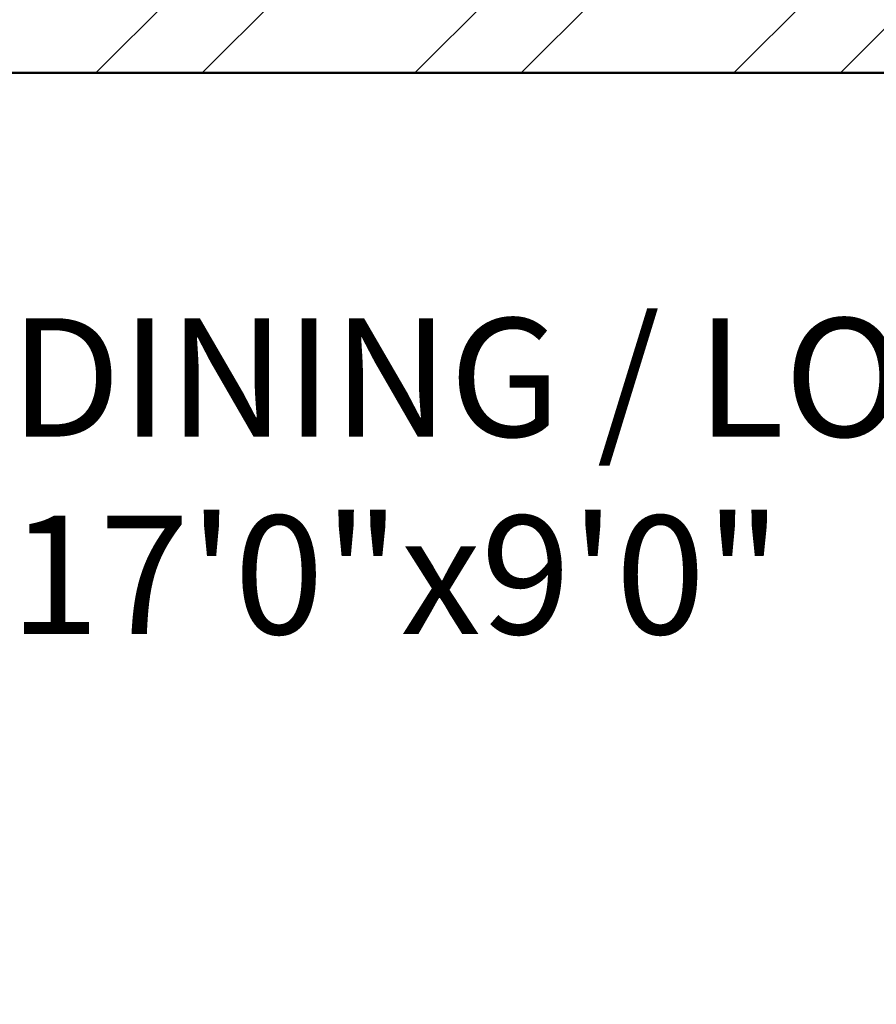
# Model space of a CAD drawing. Units: inches. Extents: x 963 to 2075, y 289 to 2657.
# Tile 63 of 98: x 1188 to 1224, y 2284 to 2325. Entities that reach past the tile are written whole.
import ezdxf

# ---------------------------------------------------------------- set-up
doc = ezdxf.new("R2010")
doc.units = ezdxf.units.IN
for name, color, linetype, lineweight in [('A-AREA-IDEN', 7, 'Continuous', 18), ('A-WALL', 7, 'Continuous', 50), ('A-WALL-PATT', 8, 'Continuous', 13)]:
    doc.layers.add(name, color=color, linetype=linetype, lineweight=lineweight)
doc.styles.get("Standard").update_dxf_attribs({"font": 'arial.ttf'})

msp = doc.modelspace()

# ---------------------------------------------------------------- hatches: boundary and pattern name
at = {"layer": 'A-WALL-PATT'}
h = msp.add_hatch(dxfattribs=at)
h.set_pattern_fill('ANSI32', color=256)
h.paths.add_polyline_path([(1296.922, 2558.318), (1203.922, 2558.318), (1203.922, 2493.818), (1191.533, 2493.818), (1191.533, 2489.318), (1211.063, 2489.318), (1211.063, 2492.02), (1211.063, 2493.818), (1208.422, 2493.818), (1208.422, 2553.818), (1292.422, 2553.818), (1292.422, 2538.863), (1296.922, 2538.863)])
h.paths.add_polyline_path([(1442.422, 2558.318), (1349.422, 2558.318), (1349.422, 2538.943), (1353.922, 2538.943), (1353.922, 2553.818), (1437.922, 2553.818), (1437.922, 2493.818), (1434.542, 2493.818), (1434.542, 2489.318), (1448.311, 2489.318), (1448.311, 2491.568), (1448.311, 2493.818), (1442.422, 2493.818)])
h.paths.add_polyline_path([(1415.554, 2491.568), (1415.554, 2493.818), (1340.941, 2493.818), (1340.941, 2489.318), (1371.922, 2489.318), (1371.922, 2378.318), (1367.596, 2378.318), (1367.596, 2373.818), (1371.922, 2373.818), (1371.922, 2355.185), (1376.422, 2355.185), (1376.422, 2489.318), (1415.554, 2489.318)])
h.paths.add_polyline_path([(1304.941, 2491.568), (1304.941, 2493.818), (1296.922, 2493.818), (1296.922, 2514.863), (1292.422, 2514.863), (1292.422, 2493.818), (1232.808, 2493.818), (1232.808, 2489.318), (1256.422, 2489.318), (1256.422, 2327.318), (1253.714, 2327.318), (1253.714, 2322.818), (1328.422, 2322.818), (1328.422, 2331.147), (1323.922, 2331.147), (1323.922, 2327.318), (1260.922, 2327.318), (1260.922, 2373.818), (1323.922, 2373.818), (1323.922, 2357.812), (1328.422, 2357.812), (1328.422, 2373.818), (1346.007, 2373.818), (1346.007, 2376.068), (1346.007, 2378.318), (1260.922, 2378.318), (1260.922, 2489.318), (1304.941, 2489.318)])
h.paths.add_polyline_path([(1226.654, 2327.318), (1124.422, 2327.318), (1124.422, 2347.447), (1119.922, 2347.447), (1119.922, 2322.818), (1163.422, 2322.818), (1163.422, 2305.435), (1165.672, 2305.435), (1167.922, 2305.435), (1167.922, 2322.818), (1226.654, 2322.818), (1226.654, 2325.068)])
h.paths.add_polyline_path([(1095.922, 2489.318), (1124.422, 2489.318), (1131.533, 2489.318), (1131.533, 2491.568), (1131.533, 2493.818), (1119.922, 2493.818), (1091.422, 2493.818), (1091.422, 2417.318), (1095.922, 2417.318), (1119.922, 2417.318), (1119.922, 2407.447), (1124.422, 2407.447), (1124.422, 2421.818), (1095.922, 2421.818)])
h.paths.add_polyline_path([(1512.922, 2558.318), (1508.422, 2558.318), (1508.422, 2493.818), (1503.401, 2493.818), (1503.401, 2489.318), (1508.422, 2489.318), (1508.422, 2327.318), (1376.422, 2327.318), (1376.422, 2330.273), (1371.922, 2330.273), (1371.922, 2298.744), (1376.422, 2298.744), (1376.422, 2322.818), (1508.422, 2322.818), (1508.422, 2165.318), (1504.255, 2165.318), (1504.255, 2160.818), (1508.422, 2160.818), (1508.422, 2108.318), (1512.922, 2108.318), (1512.922, 2160.818), (1516.182, 2160.818), (1516.182, 2163.068), (1516.182, 2165.318), (1512.922, 2165.318), (1512.922, 2322.818), (1644.922, 2322.818), (1644.922, 2298.744), (1649.422, 2298.744), (1649.422, 2322.818), (1649.422, 2330.944), (1647.172, 2330.944), (1644.922, 2330.944), (1644.922, 2327.318), (1512.922, 2327.318), (1512.922, 2489.318), (1516.759, 2489.318), (1516.759, 2491.568), (1516.759, 2493.818), (1512.922, 2493.818)])
h.paths.add_polyline_path([(1671.922, 2558.318), (1578.922, 2558.318), (1578.922, 2493.818), (1573.526, 2493.818), (1573.526, 2489.318), (1586.537, 2489.318), (1586.537, 2491.568), (1586.537, 2493.818), (1583.422, 2493.818), (1583.422, 2553.818), (1667.422, 2553.818), (1667.422, 2541.109), (1671.922, 2541.109)])
h.paths.add_polyline_path([(1681.257, 2493.818), (1671.922, 2493.818), (1671.922, 2517.109), (1667.422, 2517.109), (1667.422, 2493.818), (1610.218, 2493.818), (1610.218, 2489.318), (1644.922, 2489.318), (1644.922, 2357.865), (1649.422, 2357.865), (1649.422, 2373.818), (1652.203, 2373.818), (1652.203, 2375.827), (1652.203, 2378.318), (1649.422, 2378.318), (1649.422, 2489.318), (1681.257, 2489.318), (1681.257, 2491.568)])
h.paths.add_polyline_path([(1821.922, 2558.318), (1728.922, 2558.318), (1728.922, 2541), (1733.422, 2541), (1733.422, 2553.818), (1817.422, 2553.818), (1817.422, 2493.818), (1813.507, 2493.818), (1813.507, 2489.318), (1830.078, 2489.318), (1830.078, 2491.568), (1830.078, 2493.818), (1821.922, 2493.818)])
h.paths.add_polyline_path([(1794.244, 2493.818), (1717.257, 2493.818), (1717.257, 2489.318), (1760.422, 2489.318), (1760.422, 2378.318), (1674.401, 2378.318), (1674.401, 2373.818), (1692.922, 2373.818), (1692.922, 2356.954), (1697.422, 2356.954), (1697.422, 2373.818), (1760.422, 2373.818), (1760.422, 2327.318), (1697.422, 2327.318), (1697.422, 2333.341), (1692.922, 2333.341), (1692.922, 2322.818), (1768.037, 2322.818), (1768.037, 2325.068), (1768.037, 2327.318), (1764.922, 2327.318), (1764.922, 2489.318), (1794.244, 2489.318)])
h.paths.add_polyline_path([(1733.422, 2517), (1728.922, 2517), (1728.922, 2493.818), (1733.422, 2493.818)], flags=17)
h.paths.add_polyline_path([(1929.922, 2493.818), (1890.078, 2493.818), (1890.078, 2489.318), (1896.922, 2489.318), (1925.422, 2489.318), (1925.422, 2421.818), (1896.922, 2421.818), (1896.922, 2408.318), (1901.422, 2408.318), (1901.422, 2417.318), (1925.422, 2417.318), (1929.922, 2417.318)])
h.paths.add_polyline_path([(1901.422, 2348.318), (1896.922, 2348.318), (1896.922, 2327.318), (1800.423, 2327.318), (1800.423, 2322.818), (1853.422, 2322.818), (1853.422, 2309.453), (1857.922, 2309.453), (1857.922, 2322.818), (1901.422, 2322.818)])
h.paths.add_polyline_path([(1857.922, 2249.453), (1853.422, 2249.453), (1853.422, 2214.818), (1686.309, 2214.818), (1686.309, 2210.318), (1853.422, 2210.318), (1853.422, 2202.134), (1857.922, 2202.134), (1857.922, 2210.318)])
h.paths.add_polyline_path([(1857.922, 2142.134), (1853.422, 2142.134), (1853.422, 2115.422), (1841.422, 2115.422), (1841.422, 2088.531), (1841.422, 2046.949), (1845.922, 2046.949), (1845.922, 2110.922), (1905.922, 2110.922), (1905.922, 2092.517), (1910.422, 2092.517), (1910.422, 2115.422), (1857.922, 2115.422)])
h.paths.add_polyline_path([(1532.436, 1482.342), (1573.456, 1482.342), (1573.456, 1501), (1532.436, 1501)], flags=9)
h.paths.add_polyline_path([(1438.658, 1486.302), (1479.678, 1486.302), (1479.678, 1504.96), (1438.658, 1504.96)], flags=9)
h.paths.add_polyline_path([(1411.215, 1365.308), (1659.139, 1365.308), (1659.139, 1402.401), (1411.215, 1402.401)], flags=9)
h.paths.add_polyline_path([(1185.671, 2296.298), (1248.16, 2296.298), (1248.16, 2314.955), (1185.671, 2314.955)], flags=9)
h.paths.add_polyline_path([(1177.31, 2187.35), (1216.15, 2187.35), (1216.15, 2206.007), (1177.31, 2206.007)], flags=9)
h.paths.add_polyline_path([(1295.101, 1602.083), (1328.26, 1602.083), (1328.26, 1620.741), (1295.101, 1620.741)], flags=9)
h.paths.add_polyline_path([(1525.126, 2005.99), (1558.39, 2005.99), (1558.39, 2024.648), (1525.126, 2024.648)], flags=9)
h.paths.add_polyline_path([(1459.606, 1977.125), (1472.195, 1977.125), (1472.195, 1987.429), (1459.606, 1987.429)], flags=9)
h.paths.add_polyline_path([(1467.815, 2053.676), (1480.018, 2053.676), (1480.018, 2063.979), (1467.815, 2063.979)], flags=9)
h.paths.add_polyline_path([(1555.184, 2119.02), (1584.563, 2119.02), (1584.563, 2137.678), (1555.184, 2137.678)], flags=25)
h.paths.add_polyline_path([(1405.389, 2115.291), (1444.478, 2115.291), (1444.478, 2133.948), (1405.389, 2133.948)], flags=25)
h.paths.add_polyline_path([(1698.482, 2004.259), (1727.695, 2004.259), (1727.695, 2022.916), (1698.482, 2022.916)], flags=9)
h.paths.add_polyline_path([(1612.158, 1972.855), (1629.016, 1972.855), (1629.016, 1983.159), (1612.158, 1983.159)], flags=9)
h.paths.add_polyline_path([(1608.289, 2060.036), (1625.147, 2060.036), (1625.147, 2070.34), (1608.289, 2070.34)], flags=9)
h.paths.add_polyline_path([(1527.954, 1684.402), (1566.795, 1684.402), (1566.795, 1703.06), (1527.954, 1703.06)], flags=9)
h.paths.add_polyline_path([(1422.792, 1683.59), (1461.633, 1683.59), (1461.633, 1702.247), (1422.792, 1702.247)], flags=9)
h.paths.add_polyline_path([(1531.262, 1732.459), (1574.015, 1732.459), (1574.015, 1751.116), (1531.262, 1751.116)], flags=9)
h.paths.add_polyline_path([(1402.872, 1732.845), (1439.799, 1732.845), (1439.799, 1751.502), (1402.872, 1751.502)], flags=9)
h.paths.add_polyline_path([(1243.122, 1923.132), (1281.962, 1923.132), (1281.962, 1941.79), (1243.122, 1941.79)], flags=9)
h.paths.add_polyline_path([(1181.752, 1792.268), (1244.241, 1792.268), (1244.241, 1810.926), (1181.752, 1810.926)], flags=9)
h.paths.add_polyline_path([(1265.822, 1670.3), (1316.071, 1670.3), (1316.071, 1688.957), (1265.822, 1688.957)], flags=9)
h.paths.add_polyline_path([(1140.263, 1676.054), (1179.104, 1676.054), (1179.104, 1694.711), (1140.263, 1694.711)], flags=9)
h.paths.add_polyline_path([(1107.49, 1490.889), (1143.374, 1490.889), (1143.374, 1509.546), (1107.49, 1509.546)], flags=9)
h.paths.add_polyline_path([(1217.584, 1483.899), (1246.741, 1483.899), (1246.741, 1502.556), (1217.584, 1502.556)], flags=9)
h.paths.add_polyline_path([(1389.21, 1486.919), (1418.367, 1486.919), (1418.367, 1505.576), (1389.21, 1505.576)], flags=9)
h.paths.add_polyline_path([(1672.208, 1602.083), (1705.366, 1602.083), (1705.366, 1620.741), (1672.208, 1620.741)], flags=9)
h.paths.add_polyline_path([(1752.082, 1522.638), (1781.24, 1522.638), (1781.24, 1541.295), (1752.082, 1541.295)], flags=9)
h.paths.add_polyline_path([(1848.275, 1491.26), (1884.158, 1491.26), (1884.158, 1509.918), (1848.275, 1509.918)], flags=9)
h.paths.add_polyline_path([(1822.47, 1685.62), (1861.31, 1685.62), (1861.31, 1704.278), (1822.47, 1704.278)], flags=9)
h.paths.add_polyline_path([(1713.195, 1672.232), (1763.444, 1672.232), (1763.444, 1690.889), (1713.195, 1690.889)], flags=9)
h.paths.add_polyline_path([(1736.619, 1790.578), (1799.109, 1790.578), (1799.109, 1809.235), (1736.619, 1809.235)], flags=9)
h.paths.add_polyline_path([(1691.491, 1916.355), (1730.332, 1916.355), (1730.332, 1935.013), (1691.491, 1935.013)], flags=9)
h.paths.add_polyline_path([(1764.872, 1973.922), (1794.306, 1973.922), (1794.306, 1992.58), (1764.872, 1992.58)], flags=9)
h.paths.add_polyline_path([(1767.854, 2034.017), (1797.288, 2034.017), (1797.288, 2052.674), (1767.854, 2052.674)], flags=9)
h.paths.add_polyline_path([(1851.593, 2060.331), (1880.751, 2060.331), (1880.751, 2078.989), (1851.593, 2078.989)], flags=25)
h.paths.add_polyline_path([(1688.491, 2086.874), (1727.332, 2086.874), (1727.332, 2105.531), (1688.491, 2105.531)], flags=9)
h.paths.add_polyline_path([(1537.743, 2293.581), (1580.495, 2293.581), (1580.495, 2312.239), (1537.743, 2312.239)], flags=25)
h.paths.add_polyline_path([(1425.587, 2296.109), (1468.34, 2296.109), (1468.34, 2314.766), (1425.587, 2314.766)], flags=25)
h.paths.add_polyline_path([(1278.518, 2004.184), (1307.72, 2004.184), (1307.72, 2022.841), (1278.518, 2022.841)], flags=9)
h.paths.add_polyline_path([(1193.282, 1973.635), (1222.715, 1973.635), (1222.715, 1992.292), (1193.282, 1992.292)], flags=9)
h.paths.add_polyline_path([(1192.411, 2040.577), (1221.845, 2040.577), (1221.845, 2059.234), (1192.411, 2059.234)], flags=9)
h.paths.add_polyline_path([(1130.603, 1951.393), (1159.76, 1951.393), (1159.76, 1970.05), (1130.603, 1970.05)], flags=9)
h.paths.add_polyline_path([(1132.827, 2052.494), (1161.984, 2052.494), (1161.984, 2071.151), (1132.827, 2071.151)], flags=9)
h.paths.add_polyline_path([(1265.128, 2334.619), (1315.377, 2334.619), (1315.377, 2353.277), (1265.128, 2353.277)], flags=25)
h.paths.add_polyline_path([(1136.741, 2330.785), (1175.582, 2330.785), (1175.582, 2349.443), (1136.741, 2349.443)], flags=9)
h.paths.add_polyline_path([(1287.422, 2417.204), (1320.58, 2417.204), (1320.58, 2435.861), (1287.422, 2435.861)], flags=25)
h.paths.add_polyline_path([(1430.988, 2329.159), (1469.828, 2329.159), (1469.828, 2347.816), (1430.988, 2347.816)], flags=25)
h.paths.add_polyline_path([(1525.424, 2329.213), (1564.264, 2329.213), (1564.264, 2347.87), (1525.424, 2347.87)], flags=25)
h.paths.add_polyline_path([(1684.525, 2382.799), (1717.683, 2382.799), (1717.683, 2401.457), (1684.525, 2401.457)], flags=25)
h.paths.add_polyline_path([(1704.805, 2340.293), (1755.054, 2340.293), (1755.054, 2358.95), (1704.805, 2358.95)], flags=25)
h.paths.add_polyline_path([(1694.113, 2287.757), (1756.602, 2287.757), (1756.602, 2306.414), (1694.113, 2306.414)], flags=9)
h.paths.add_polyline_path([(1815.778, 2329.861), (1854.618, 2329.861), (1854.618, 2348.518), (1815.778, 2348.518)], flags=9)
h.paths.add_polyline_path([(1842.873, 2514.256), (1878.756, 2514.256), (1878.756, 2532.914), (1842.873, 2532.914)], flags=9)
h.paths.add_polyline_path([(1769.513, 2531.447), (1798.671, 2531.447), (1798.671, 2550.104), (1769.513, 2550.104)], flags=25)
h.paths.add_polyline_path([(1594.772, 2518.468), (1623.93, 2518.468), (1623.93, 2537.125), (1594.772, 2537.125)], flags=25)
h.paths.add_polyline_path([(1520.723, 2516.185), (1556.606, 2516.185), (1556.606, 2534.842), (1520.723, 2534.842)], flags=25)
h.paths.add_polyline_path([(1464.456, 2516.694), (1500.34, 2516.694), (1500.34, 2535.351), (1464.456, 2535.351)], flags=25)
h.paths.add_polyline_path([(1365.696, 2528.97), (1394.854, 2528.97), (1394.854, 2547.627), (1365.696, 2547.627)], flags=25)
h.paths.add_polyline_path([(1222.838, 2516.231), (1251.995, 2516.231), (1251.995, 2534.889), (1222.838, 2534.889)], flags=25)
h.paths.add_polyline_path([(1104.545, 2509.6), (1140.429, 2509.6), (1140.429, 2528.257), (1104.545, 2528.257)], flags=9)
h = msp.add_hatch(dxfattribs=at)
h.set_pattern_fill('ANSI32', color=256)
h.paths.add_polyline_path([(1335.968, 2212.568), (1335.968, 2214.818), (1167.922, 2214.818), (1167.922, 2245.435), (1163.422, 2245.435), (1163.422, 2210.318), (1163.422, 2194.812), (1167.922, 2194.812), (1167.922, 2210.318), (1335.968, 2210.318)])
h.paths.add_polyline_path([(1532.436, 1482.342), (1573.456, 1482.342), (1573.456, 1501), (1532.436, 1501)], flags=9)
h.paths.add_polyline_path([(1438.658, 1486.302), (1479.678, 1486.302), (1479.678, 1504.96), (1438.658, 1504.96)], flags=9)
h.paths.add_polyline_path([(1411.215, 1365.308), (1659.139, 1365.308), (1659.139, 1402.401), (1411.215, 1402.401)], flags=9)
h.paths.add_polyline_path([(1185.671, 2296.298), (1248.16, 2296.298), (1248.16, 2314.955), (1185.671, 2314.955)], flags=9)
h.paths.add_polyline_path([(1177.31, 2187.35), (1216.15, 2187.35), (1216.15, 2206.007), (1177.31, 2206.007)], flags=9)
h.paths.add_polyline_path([(1295.101, 1602.083), (1328.26, 1602.083), (1328.26, 1620.741), (1295.101, 1620.741)], flags=9)
h.paths.add_polyline_path([(1525.126, 2005.99), (1558.39, 2005.99), (1558.39, 2024.648), (1525.126, 2024.648)], flags=9)
h.paths.add_polyline_path([(1459.606, 1977.125), (1472.195, 1977.125), (1472.195, 1987.429), (1459.606, 1987.429)], flags=9)
h.paths.add_polyline_path([(1467.815, 2053.676), (1480.018, 2053.676), (1480.018, 2063.979), (1467.815, 2063.979)], flags=9)
h.paths.add_polyline_path([(1555.184, 2119.02), (1584.563, 2119.02), (1584.563, 2137.678), (1555.184, 2137.678)], flags=9)
h.paths.add_polyline_path([(1405.389, 2115.291), (1444.478, 2115.291), (1444.478, 2133.948), (1405.389, 2133.948)], flags=9)
h.paths.add_polyline_path([(1698.482, 2004.259), (1727.695, 2004.259), (1727.695, 2022.916), (1698.482, 2022.916)], flags=9)
h.paths.add_polyline_path([(1612.158, 1972.855), (1629.016, 1972.855), (1629.016, 1983.159), (1612.158, 1983.159)], flags=9)
h.paths.add_polyline_path([(1608.289, 2060.036), (1625.147, 2060.036), (1625.147, 2070.34), (1608.289, 2070.34)], flags=9)
h.paths.add_polyline_path([(1527.954, 1684.402), (1566.795, 1684.402), (1566.795, 1703.06), (1527.954, 1703.06)], flags=9)
h.paths.add_polyline_path([(1422.792, 1683.59), (1461.633, 1683.59), (1461.633, 1702.247), (1422.792, 1702.247)], flags=9)
h.paths.add_polyline_path([(1531.262, 1732.459), (1574.015, 1732.459), (1574.015, 1751.116), (1531.262, 1751.116)], flags=9)
h.paths.add_polyline_path([(1402.872, 1732.845), (1439.799, 1732.845), (1439.799, 1751.502), (1402.872, 1751.502)], flags=9)
h.paths.add_polyline_path([(1243.122, 1923.132), (1281.962, 1923.132), (1281.962, 1941.79), (1243.122, 1941.79)], flags=9)
h.paths.add_polyline_path([(1181.752, 1792.268), (1244.241, 1792.268), (1244.241, 1810.926), (1181.752, 1810.926)], flags=9)
h.paths.add_polyline_path([(1265.822, 1670.3), (1316.071, 1670.3), (1316.071, 1688.957), (1265.822, 1688.957)], flags=9)
h.paths.add_polyline_path([(1140.263, 1676.054), (1179.104, 1676.054), (1179.104, 1694.711), (1140.263, 1694.711)], flags=9)
h.paths.add_polyline_path([(1107.49, 1490.889), (1143.374, 1490.889), (1143.374, 1509.546), (1107.49, 1509.546)], flags=9)
h.paths.add_polyline_path([(1217.584, 1483.899), (1246.741, 1483.899), (1246.741, 1502.556), (1217.584, 1502.556)], flags=9)
h.paths.add_polyline_path([(1389.21, 1486.919), (1418.367, 1486.919), (1418.367, 1505.576), (1389.21, 1505.576)], flags=9)
h.paths.add_polyline_path([(1672.208, 1602.083), (1705.366, 1602.083), (1705.366, 1620.741), (1672.208, 1620.741)], flags=9)
h.paths.add_polyline_path([(1752.082, 1522.638), (1781.24, 1522.638), (1781.24, 1541.295), (1752.082, 1541.295)], flags=9)
h.paths.add_polyline_path([(1848.275, 1491.26), (1884.158, 1491.26), (1884.158, 1509.918), (1848.275, 1509.918)], flags=9)
h.paths.add_polyline_path([(1822.47, 1685.62), (1861.31, 1685.62), (1861.31, 1704.278), (1822.47, 1704.278)], flags=9)
h.paths.add_polyline_path([(1713.195, 1672.232), (1763.444, 1672.232), (1763.444, 1690.889), (1713.195, 1690.889)], flags=9)
h.paths.add_polyline_path([(1736.619, 1790.578), (1799.109, 1790.578), (1799.109, 1809.235), (1736.619, 1809.235)], flags=9)
h.paths.add_polyline_path([(1691.491, 1916.355), (1730.332, 1916.355), (1730.332, 1935.013), (1691.491, 1935.013)], flags=9)
h.paths.add_polyline_path([(1764.872, 1973.922), (1794.306, 1973.922), (1794.306, 1992.58), (1764.872, 1992.58)], flags=9)
h.paths.add_polyline_path([(1767.854, 2034.017), (1797.288, 2034.017), (1797.288, 2052.674), (1767.854, 2052.674)], flags=9)
h.paths.add_polyline_path([(1851.593, 2060.331), (1880.751, 2060.331), (1880.751, 2078.989), (1851.593, 2078.989)], flags=9)
h.paths.add_polyline_path([(1688.491, 2086.874), (1727.332, 2086.874), (1727.332, 2105.531), (1688.491, 2105.531)], flags=9)
h.paths.add_polyline_path([(1537.743, 2293.581), (1580.495, 2293.581), (1580.495, 2312.239), (1537.743, 2312.239)], flags=9)
h.paths.add_polyline_path([(1425.587, 2296.109), (1468.34, 2296.109), (1468.34, 2314.766), (1425.587, 2314.766)], flags=9)
h.paths.add_polyline_path([(1278.518, 2004.184), (1307.72, 2004.184), (1307.72, 2022.841), (1278.518, 2022.841)], flags=9)
h.paths.add_polyline_path([(1193.282, 1973.635), (1222.715, 1973.635), (1222.715, 1992.292), (1193.282, 1992.292)], flags=9)
h.paths.add_polyline_path([(1192.411, 2040.577), (1221.845, 2040.577), (1221.845, 2059.234), (1192.411, 2059.234)], flags=9)
h.paths.add_polyline_path([(1130.603, 1951.393), (1159.76, 1951.393), (1159.76, 1970.05), (1130.603, 1970.05)], flags=9)
h.paths.add_polyline_path([(1132.827, 2052.494), (1161.984, 2052.494), (1161.984, 2071.151), (1132.827, 2071.151)], flags=9)
h.paths.add_polyline_path([(1265.128, 2334.619), (1315.377, 2334.619), (1315.377, 2353.277), (1265.128, 2353.277)], flags=9)
h.paths.add_polyline_path([(1136.741, 2330.785), (1175.582, 2330.785), (1175.582, 2349.443), (1136.741, 2349.443)], flags=9)
h.paths.add_polyline_path([(1287.422, 2417.204), (1320.58, 2417.204), (1320.58, 2435.861), (1287.422, 2435.861)], flags=9)
h.paths.add_polyline_path([(1430.988, 2329.159), (1469.828, 2329.159), (1469.828, 2347.816), (1430.988, 2347.816)], flags=9)
h.paths.add_polyline_path([(1525.424, 2329.213), (1564.264, 2329.213), (1564.264, 2347.87), (1525.424, 2347.87)], flags=9)
h.paths.add_polyline_path([(1684.525, 2382.799), (1717.683, 2382.799), (1717.683, 2401.457), (1684.525, 2401.457)], flags=9)
h.paths.add_polyline_path([(1704.805, 2340.293), (1755.054, 2340.293), (1755.054, 2358.95), (1704.805, 2358.95)], flags=9)
h.paths.add_polyline_path([(1694.113, 2287.757), (1756.602, 2287.757), (1756.602, 2306.414), (1694.113, 2306.414)], flags=9)
h.paths.add_polyline_path([(1815.778, 2329.861), (1854.618, 2329.861), (1854.618, 2348.518), (1815.778, 2348.518)], flags=9)
h.paths.add_polyline_path([(1842.873, 2514.256), (1878.756, 2514.256), (1878.756, 2532.914), (1842.873, 2532.914)], flags=9)
h.paths.add_polyline_path([(1769.513, 2531.447), (1798.671, 2531.447), (1798.671, 2550.104), (1769.513, 2550.104)], flags=9)
h.paths.add_polyline_path([(1594.772, 2518.468), (1623.93, 2518.468), (1623.93, 2537.125), (1594.772, 2537.125)], flags=9)
h.paths.add_polyline_path([(1520.723, 2516.185), (1556.606, 2516.185), (1556.606, 2534.842), (1520.723, 2534.842)], flags=9)
h.paths.add_polyline_path([(1464.456, 2516.694), (1500.34, 2516.694), (1500.34, 2535.351), (1464.456, 2535.351)], flags=9)
h.paths.add_polyline_path([(1365.696, 2528.97), (1394.854, 2528.97), (1394.854, 2547.627), (1365.696, 2547.627)], flags=9)
h.paths.add_polyline_path([(1222.838, 2516.231), (1251.995, 2516.231), (1251.995, 2534.889), (1222.838, 2534.889)], flags=9)
h.paths.add_polyline_path([(1104.545, 2509.6), (1140.429, 2509.6), (1140.429, 2528.257), (1104.545, 2528.257)], flags=9)

# ---------------------------------------------------------------- linework, layer by layer
at = {"layer": 'A-WALL'}
msp.add_line((1167.922, 2322.818), (1226.654, 2322.818), dxfattribs=at)

# ---------------------------------------------------------------- texts
at = {"layer": 'A-AREA-IDEN', "insert": (1187.681, 2312.47), "char_height": 5, "attachment_point": 1}
msp.add_mtext_dynamic_manual_height_columns('DINING / LOUNGE\\P17\'0"x9\'0"', width=166.99497, gutter_width=12.5, heights=[0], dxfattribs=at)

doc.saveas('drawing.dxf')
